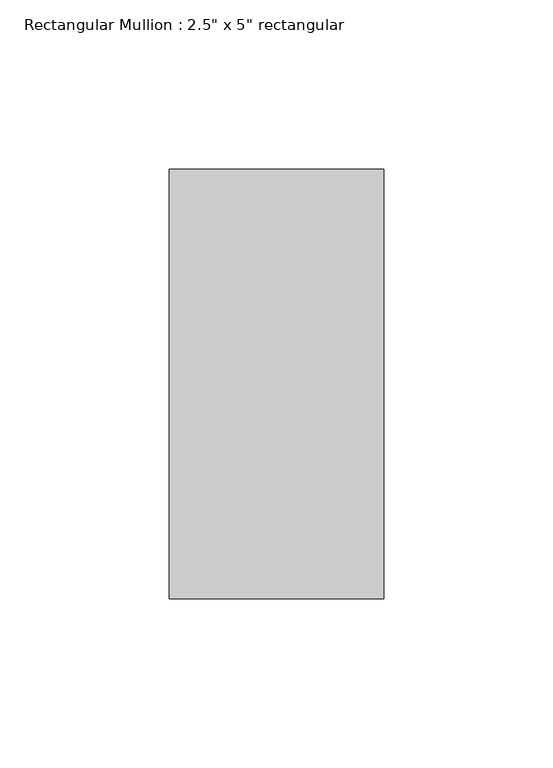
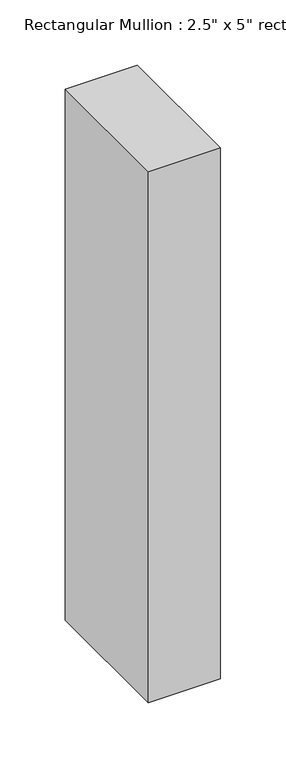
"""IFC4 building model written with IfcOpenShell, lengths in millimetres: member geometry."""

from ifc_helpers import new_model, si_unit, frame, origin, place, context, project, spatial, polyline, outline, extrude, source, transform, mapped, element, save


def member_2ebf4a73(model_context):
    return source(origin(), model_context, "Body", "SweptSolid", [
        extrude(outline(polyline([(0.0, 63.5), (0.0, -63.5), (-63.5, -63.5), (-63.5, 63.5), (0.0, 63.5)])), frame((0.0, 0.0, -495.3), z_axis=(0.0, 0.0, 1.0), x_axis=(1.0, 0.0, 0.0)), (0.0, 0.0, 1.0), 495.3),
    ])


if __name__ == "__main__":
    model = new_model("IFC4")
    model_context = context("Model", 3, world=origin())
    ifc_project = project(units=[si_unit("LENGTHUNIT", "METRE", prefix="MILLI")], contexts=[model_context])
    site = spatial("IfcSite", under=ifc_project)
    building = spatial("IfcBuilding", under=site)
    placement = place(None, origin())
    member_shape = member_2ebf4a73(model_context)
    element("IfcMember", 1, ObjectType="Rectangular Mullion : 2.5\" x 5\" rectangular", at=placement, inside=building, context=model_context, shape_type="MappedRepresentation", body=[
        mapped(member_shape, transform((0.0, 0.0, 0.0), x_axis=(1.0, 0.0, 0.0), y_axis=(0.0, 1.0, 0.0), z_axis=(0.0, 0.0, 1.0))),
    ])
    save(model, "model.ifc")

# Revit data of these elements
# Type "Rectangular Mullion : 2.5\" x 5\" rectangular"
#   built-in parameter 1007304 = 0.416667 (stored number, unit not read)
#   built-in parameter 1007301 = 0.104167 (stored number, unit not read)
#   built-in parameter 1007300 = 0.104167 (stored number, unit not read)
# Element 1 (IfcMember, "Rectangular Mullion : 2.5\" x 5\" rectangular")
#   Materials on its faces: "Aluminum"
# Materials
#   "Aluminum": class "Metal", colour RGB 247 247 247, transparency 0, Description = "Aluminum 6061", Cost = 0
